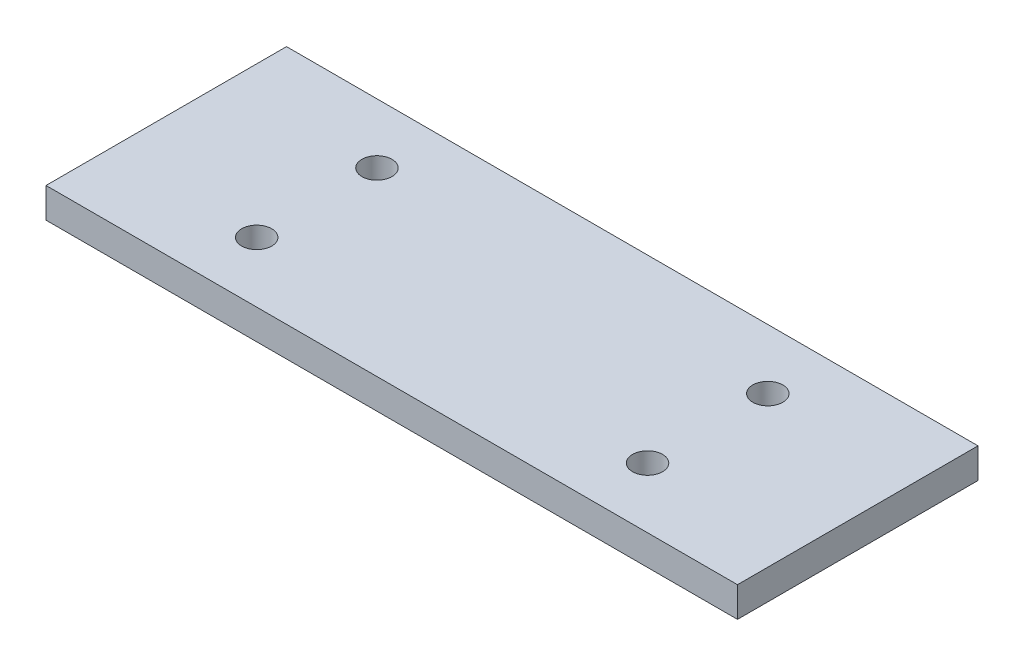
ISO-10303-21;
HEADER;
FILE_DESCRIPTION(('STEP AP214'),'2;1');
FILE_NAME('part.step','',(''),(''),'','','');
FILE_SCHEMA(('AUTOMOTIVE_DESIGN { 1 0 10303 214 1 1 1 1 }'));
ENDSEC;
DATA;
#1=APPLICATION_CONTEXT('core data for automotive mechanical design processes');
#2=APPLICATION_PROTOCOL_DEFINITION('international standard','automotive_design',2000,#1);
#3=PRODUCT_CONTEXT('',#1,'mechanical');
#4=PRODUCT('Part','Part','',(#3));
#5=PRODUCT_RELATED_PRODUCT_CATEGORY('part','',(#4));
#6=PRODUCT_DEFINITION_FORMATION('','',#4);
#7=PRODUCT_DEFINITION_CONTEXT('part definition',#1,'design');
#8=PRODUCT_DEFINITION('design','',#6,#7);
#9=PRODUCT_DEFINITION_SHAPE('','',#8);
#10=(LENGTH_UNIT() NAMED_UNIT(*) SI_UNIT(.MILLI.,.METRE.));
#11=(NAMED_UNIT(*) PLANE_ANGLE_UNIT() SI_UNIT($,.RADIAN.));
#12=(NAMED_UNIT(*) SI_UNIT($,.STERADIAN.) SOLID_ANGLE_UNIT());
#13=UNCERTAINTY_MEASURE_WITH_UNIT(LENGTH_MEASURE(1.E-05),#10,'distance_accuracy_value','');
#14=(GEOMETRIC_REPRESENTATION_CONTEXT(3) GLOBAL_UNCERTAINTY_ASSIGNED_CONTEXT((#13)) GLOBAL_UNIT_ASSIGNED_CONTEXT((#10,
#11,#12)) REPRESENTATION_CONTEXT('',''));
#15=CARTESIAN_POINT('',(0.,0.,0.));
#16=DIRECTION('',(0.,0.,1.));
#17=DIRECTION('',(1.,0.,0.));
#18=AXIS2_PLACEMENT_3D('',#15,#16,#17);
#19=CARTESIAN_POINT('',(0.,5.,0.));
#20=DIRECTION('',(0.,1.,0.));
#21=DIRECTION('',(0.,0.,1.));
#22=AXIS2_PLACEMENT_3D('',#19,#20,#21);
#23=PLANE('',#22);
#24=CARTESIAN_POINT('',(32.5,5.,9.95863970588235));
#25=DIRECTION('',(0.,1.,0.));
#26=DIRECTION('',(0.,0.,-1.));
#27=AXIS2_PLACEMENT_3D('',#24,#25,#26);
#28=CIRCLE('',#27,2.5);
#29=CARTESIAN_POINT('',(32.5,5.,7.45863970588235));
#30=VERTEX_POINT('',#29);
#31=EDGE_CURVE('E130',#30,#30,#28,.T.);
#32=ORIENTED_EDGE('',*,*,#31,.F.);
#33=EDGE_LOOP('',(#32));
#34=FACE_BOUND('',#33,.T.);
#35=CARTESIAN_POINT('',(-32.5,5.,-10.0413602941176));
#36=DIRECTION('',(0.,1.,0.));
#37=DIRECTION('',(0.,0.,1.));
#38=AXIS2_PLACEMENT_3D('',#35,#36,#37);
#39=CIRCLE('',#38,2.5);
#40=CARTESIAN_POINT('',(-32.5,5.,-7.54136029411765));
#41=VERTEX_POINT('',#40);
#42=EDGE_CURVE('E106',#41,#41,#39,.T.);
#43=ORIENTED_EDGE('',*,*,#42,.F.);
#44=EDGE_LOOP('',(#43));
#45=FACE_BOUND('',#44,.T.);
#46=DIRECTION('',(0.,0.,-1.));
#47=VECTOR('',#46,1.);
#48=CARTESIAN_POINT('',(57.5,5.,-20.));
#49=LINE('',#48,#47);
#50=CARTESIAN_POINT('',(57.5,5.,20.));
#51=VERTEX_POINT('',#50);
#52=CARTESIAN_POINT('',(57.5,5.,-20.));
#53=VERTEX_POINT('',#52);
#54=EDGE_CURVE('E93',#51,#53,#49,.T.);
#55=ORIENTED_EDGE('',*,*,#54,.T.);
#56=DIRECTION('',(-1.,0.,0.));
#57=VECTOR('',#56,1.);
#58=CARTESIAN_POINT('',(-57.5,5.,-20.));
#59=LINE('',#58,#57);
#60=CARTESIAN_POINT('',(-57.5,5.,-20.));
#61=VERTEX_POINT('',#60);
#62=EDGE_CURVE('E88',#53,#61,#59,.T.);
#63=ORIENTED_EDGE('',*,*,#62,.T.);
#64=DIRECTION('',(0.,0.,1.));
#65=VECTOR('',#64,1.);
#66=CARTESIAN_POINT('',(-57.5,5.,-20.));
#67=LINE('',#66,#65);
#68=CARTESIAN_POINT('',(-57.5,5.,20.));
#69=VERTEX_POINT('',#68);
#70=EDGE_CURVE('E90',#61,#69,#67,.T.);
#71=ORIENTED_EDGE('',*,*,#70,.T.);
#72=DIRECTION('',(1.,0.,0.));
#73=VECTOR('',#72,1.);
#74=CARTESIAN_POINT('',(-57.5,5.,20.));
#75=LINE('',#74,#73);
#76=EDGE_CURVE('E57',#69,#51,#75,.T.);
#77=ORIENTED_EDGE('',*,*,#76,.T.);
#78=EDGE_LOOP('',(#55,#63,#71,#77));
#79=FACE_BOUND('',#78,.T.);
#80=CARTESIAN_POINT('',(-32.5,5.,9.95863970588235));
#81=DIRECTION('',(0.,1.,0.));
#82=DIRECTION('',(0.,0.,1.));
#83=AXIS2_PLACEMENT_3D('',#80,#81,#82);
#84=CIRCLE('',#83,2.5);
#85=CARTESIAN_POINT('',(-32.5,5.,12.4586397058824));
#86=VERTEX_POINT('',#85);
#87=EDGE_CURVE('E123',#86,#86,#84,.T.);
#88=ORIENTED_EDGE('',*,*,#87,.F.);
#89=EDGE_LOOP('',(#88));
#90=FACE_BOUND('',#89,.T.);
#91=CARTESIAN_POINT('',(32.5,5.,-10.0413602941176));
#92=DIRECTION('',(0.,1.,0.));
#93=DIRECTION('',(0.,0.,-1.));
#94=AXIS2_PLACEMENT_3D('',#91,#92,#93);
#95=CIRCLE('',#94,2.5);
#96=CARTESIAN_POINT('',(32.5,5.,-12.5413602941177));
#97=VERTEX_POINT('',#96);
#98=EDGE_CURVE('E134',#97,#97,#95,.T.);
#99=ORIENTED_EDGE('',*,*,#98,.F.);
#100=EDGE_LOOP('',(#99));
#101=FACE_BOUND('',#100,.T.);
#102=ADVANCED_FACE('F39',(#34,#45,#79,#90,#101),#23,.T.);
#103=CARTESIAN_POINT('',(0.,0.,0.));
#104=DIRECTION('',(0.,1.,0.));
#105=DIRECTION('',(0.,0.,1.));
#106=AXIS2_PLACEMENT_3D('',#103,#104,#105);
#107=PLANE('',#106);
#108=DIRECTION('',(0.,0.,-1.));
#109=VECTOR('',#108,1.);
#110=CARTESIAN_POINT('',(57.5,0.,-20.));
#111=LINE('',#110,#109);
#112=CARTESIAN_POINT('',(57.5,0.,20.));
#113=VERTEX_POINT('',#112);
#114=CARTESIAN_POINT('',(57.5,0.,-20.));
#115=VERTEX_POINT('',#114);
#116=EDGE_CURVE('E103',#113,#115,#111,.T.);
#117=ORIENTED_EDGE('',*,*,#116,.F.);
#118=DIRECTION('',(1.,0.,0.));
#119=VECTOR('',#118,1.);
#120=CARTESIAN_POINT('',(-57.5,0.,20.));
#121=LINE('',#120,#119);
#122=CARTESIAN_POINT('',(-57.5,0.,20.));
#123=VERTEX_POINT('',#122);
#124=EDGE_CURVE('E76',#123,#113,#121,.T.);
#125=ORIENTED_EDGE('',*,*,#124,.F.);
#126=DIRECTION('',(0.,0.,1.));
#127=VECTOR('',#126,1.);
#128=CARTESIAN_POINT('',(-57.5,0.,-20.));
#129=LINE('',#128,#127);
#130=CARTESIAN_POINT('',(-57.5,0.,-20.));
#131=VERTEX_POINT('',#130);
#132=EDGE_CURVE('E71',#131,#123,#129,.T.);
#133=ORIENTED_EDGE('',*,*,#132,.F.);
#134=DIRECTION('',(-1.,0.,0.));
#135=VECTOR('',#134,1.);
#136=CARTESIAN_POINT('',(-57.5,0.,-20.));
#137=LINE('',#136,#135);
#138=EDGE_CURVE('E92',#115,#131,#137,.T.);
#139=ORIENTED_EDGE('',*,*,#138,.F.);
#140=EDGE_LOOP('',(#117,#125,#133,#139));
#141=FACE_BOUND('',#140,.T.);
#142=CARTESIAN_POINT('',(-32.5,0.,-10.0413602941176));
#143=DIRECTION('',(0.,1.,0.));
#144=DIRECTION('',(0.,0.,1.));
#145=AXIS2_PLACEMENT_3D('',#142,#143,#144);
#146=CIRCLE('',#145,2.5);
#147=CARTESIAN_POINT('',(-32.5,0.,-7.54136029411765));
#148=VERTEX_POINT('',#147);
#149=EDGE_CURVE('E119',#148,#148,#146,.T.);
#150=ORIENTED_EDGE('',*,*,#149,.T.);
#151=EDGE_LOOP('',(#150));
#152=FACE_BOUND('',#151,.T.);
#153=CARTESIAN_POINT('',(-32.5,0.,9.95863970588235));
#154=DIRECTION('',(0.,1.,0.));
#155=DIRECTION('',(0.,0.,1.));
#156=AXIS2_PLACEMENT_3D('',#153,#154,#155);
#157=CIRCLE('',#156,2.5);
#158=CARTESIAN_POINT('',(-32.5,0.,12.4586397058824));
#159=VERTEX_POINT('',#158);
#160=EDGE_CURVE('E122',#159,#159,#157,.T.);
#161=ORIENTED_EDGE('',*,*,#160,.T.);
#162=EDGE_LOOP('',(#161));
#163=FACE_BOUND('',#162,.T.);
#164=CARTESIAN_POINT('',(32.5,0.,9.95863970588235));
#165=DIRECTION('',(0.,1.,0.));
#166=DIRECTION('',(0.,0.,-1.));
#167=AXIS2_PLACEMENT_3D('',#164,#165,#166);
#168=CIRCLE('',#167,2.5);
#169=CARTESIAN_POINT('',(32.5,0.,7.45863970588235));
#170=VERTEX_POINT('',#169);
#171=EDGE_CURVE('E128',#170,#170,#168,.T.);
#172=ORIENTED_EDGE('',*,*,#171,.T.);
#173=EDGE_LOOP('',(#172));
#174=FACE_BOUND('',#173,.T.);
#175=CARTESIAN_POINT('',(32.5,0.,-10.0413602941176));
#176=DIRECTION('',(0.,1.,0.));
#177=DIRECTION('',(0.,0.,-1.));
#178=AXIS2_PLACEMENT_3D('',#175,#176,#177);
#179=CIRCLE('',#178,2.5);
#180=CARTESIAN_POINT('',(32.5,0.,-12.5413602941177));
#181=VERTEX_POINT('',#180);
#182=EDGE_CURVE('E138',#181,#181,#179,.T.);
#183=ORIENTED_EDGE('',*,*,#182,.T.);
#184=EDGE_LOOP('',(#183));
#185=FACE_BOUND('',#184,.T.);
#186=ADVANCED_FACE('F111',(#141,#152,#163,#174,#185),#107,.F.);
#187=CARTESIAN_POINT('',(57.5,5.,-20.));
#188=DIRECTION('',(-1.,0.,0.));
#189=DIRECTION('',(0.,0.,1.));
#190=AXIS2_PLACEMENT_3D('',#187,#188,#189);
#191=PLANE('',#190);
#192=ORIENTED_EDGE('',*,*,#116,.T.);
#193=DIRECTION('',(0.,-1.,0.));
#194=VECTOR('',#193,1.);
#195=CARTESIAN_POINT('',(57.5,5.,-20.));
#196=LINE('',#195,#194);
#197=EDGE_CURVE('E11',#53,#115,#196,.T.);
#198=ORIENTED_EDGE('',*,*,#197,.F.);
#199=ORIENTED_EDGE('',*,*,#54,.F.);
#200=DIRECTION('',(0.,-1.,0.));
#201=VECTOR('',#200,1.);
#202=CARTESIAN_POINT('',(57.5,5.,20.));
#203=LINE('',#202,#201);
#204=EDGE_CURVE('E97',#51,#113,#203,.T.);
#205=ORIENTED_EDGE('',*,*,#204,.T.);
#206=EDGE_LOOP('',(#192,#198,#199,#205));
#207=FACE_BOUND('',#206,.T.);
#208=ADVANCED_FACE('F41',(#207),#191,.F.);
#209=CARTESIAN_POINT('',(-57.5,5.,-20.));
#210=DIRECTION('',(0.,0.,1.));
#211=DIRECTION('',(1.,0.,0.));
#212=AXIS2_PLACEMENT_3D('',#209,#210,#211);
#213=PLANE('',#212);
#214=ORIENTED_EDGE('',*,*,#138,.T.);
#215=DIRECTION('',(0.,-1.,0.));
#216=VECTOR('',#215,1.);
#217=CARTESIAN_POINT('',(-57.5,5.,-20.));
#218=LINE('',#217,#216);
#219=EDGE_CURVE('E48',#61,#131,#218,.T.);
#220=ORIENTED_EDGE('',*,*,#219,.F.);
#221=ORIENTED_EDGE('',*,*,#62,.F.);
#222=ORIENTED_EDGE('',*,*,#197,.T.);
#223=EDGE_LOOP('',(#214,#220,#221,#222));
#224=FACE_BOUND('',#223,.T.);
#225=ADVANCED_FACE('F94',(#224),#213,.F.);
#226=CARTESIAN_POINT('',(-57.5,5.,-20.));
#227=DIRECTION('',(1.,0.,0.));
#228=DIRECTION('',(0.,0.,-1.));
#229=AXIS2_PLACEMENT_3D('',#226,#227,#228);
#230=PLANE('',#229);
#231=ORIENTED_EDGE('',*,*,#132,.T.);
#232=DIRECTION('',(0.,-1.,0.));
#233=VECTOR('',#232,1.);
#234=CARTESIAN_POINT('',(-57.5,5.,20.));
#235=LINE('',#234,#233);
#236=EDGE_CURVE('E96',#69,#123,#235,.T.);
#237=ORIENTED_EDGE('',*,*,#236,.F.);
#238=ORIENTED_EDGE('',*,*,#70,.F.);
#239=ORIENTED_EDGE('',*,*,#219,.T.);
#240=EDGE_LOOP('',(#231,#237,#238,#239));
#241=FACE_BOUND('',#240,.T.);
#242=ADVANCED_FACE('F100',(#241),#230,.F.);
#243=CARTESIAN_POINT('',(-57.5,5.,20.));
#244=DIRECTION('',(0.,0.,-1.));
#245=DIRECTION('',(-1.,0.,0.));
#246=AXIS2_PLACEMENT_3D('',#243,#244,#245);
#247=PLANE('',#246);
#248=ORIENTED_EDGE('',*,*,#124,.T.);
#249=ORIENTED_EDGE('',*,*,#204,.F.);
#250=ORIENTED_EDGE('',*,*,#76,.F.);
#251=ORIENTED_EDGE('',*,*,#236,.T.);
#252=EDGE_LOOP('',(#248,#249,#250,#251));
#253=FACE_BOUND('',#252,.T.);
#254=ADVANCED_FACE('F112',(#253),#247,.F.);
#255=CARTESIAN_POINT('',(-32.5,5.,-10.0413602941176));
#256=DIRECTION('',(0.,-1.,0.));
#257=DIRECTION('',(0.,0.,-1.));
#258=AXIS2_PLACEMENT_3D('',#255,#256,#257);
#259=CYLINDRICAL_SURFACE('',#258,2.5);
#260=ORIENTED_EDGE('',*,*,#42,.T.);
#261=EDGE_LOOP('',(#260));
#262=FACE_BOUND('',#261,.T.);
#263=ORIENTED_EDGE('',*,*,#149,.F.);
#264=EDGE_LOOP('',(#263));
#265=FACE_BOUND('',#264,.T.);
#266=ADVANCED_FACE('F154',(#262,#265),#259,.F.);
#267=CARTESIAN_POINT('',(-32.5,5.,9.95863970588235));
#268=DIRECTION('',(0.,-1.,0.));
#269=DIRECTION('',(0.,0.,-1.));
#270=AXIS2_PLACEMENT_3D('',#267,#268,#269);
#271=CYLINDRICAL_SURFACE('',#270,2.5);
#272=ORIENTED_EDGE('',*,*,#87,.T.);
#273=EDGE_LOOP('',(#272));
#274=FACE_BOUND('',#273,.T.);
#275=ORIENTED_EDGE('',*,*,#160,.F.);
#276=EDGE_LOOP('',(#275));
#277=FACE_BOUND('',#276,.T.);
#278=ADVANCED_FACE('F199',(#274,#277),#271,.F.);
#279=CARTESIAN_POINT('',(32.5,5.,9.95863970588235));
#280=DIRECTION('',(0.,-1.,0.));
#281=DIRECTION('',(0.,0.,-1.));
#282=AXIS2_PLACEMENT_3D('',#279,#280,#281);
#283=CYLINDRICAL_SURFACE('',#282,2.5);
#284=ORIENTED_EDGE('',*,*,#31,.T.);
#285=EDGE_LOOP('',(#284));
#286=FACE_BOUND('',#285,.T.);
#287=ORIENTED_EDGE('',*,*,#171,.F.);
#288=EDGE_LOOP('',(#287));
#289=FACE_BOUND('',#288,.T.);
#290=ADVANCED_FACE('F208',(#286,#289),#283,.F.);
#291=CARTESIAN_POINT('',(32.5,5.,-10.0413602941176));
#292=DIRECTION('',(0.,-1.,0.));
#293=DIRECTION('',(0.,0.,-1.));
#294=AXIS2_PLACEMENT_3D('',#291,#292,#293);
#295=CYLINDRICAL_SURFACE('',#294,2.5);
#296=ORIENTED_EDGE('',*,*,#98,.T.);
#297=EDGE_LOOP('',(#296));
#298=FACE_BOUND('',#297,.T.);
#299=ORIENTED_EDGE('',*,*,#182,.F.);
#300=EDGE_LOOP('',(#299));
#301=FACE_BOUND('',#300,.T.);
#302=ADVANCED_FACE('F142',(#298,#301),#295,.F.);
#303=CLOSED_SHELL('',(#102,#186,#208,#225,#242,#254,#266,#278,#290,#302));
#304=MANIFOLD_SOLID_BREP('B2',#303);
#305=ADVANCED_BREP_SHAPE_REPRESENTATION('',(#18,#304),#14);
#306=SHAPE_DEFINITION_REPRESENTATION(#9,#305);
ENDSEC;
END-ISO-10303-21;
